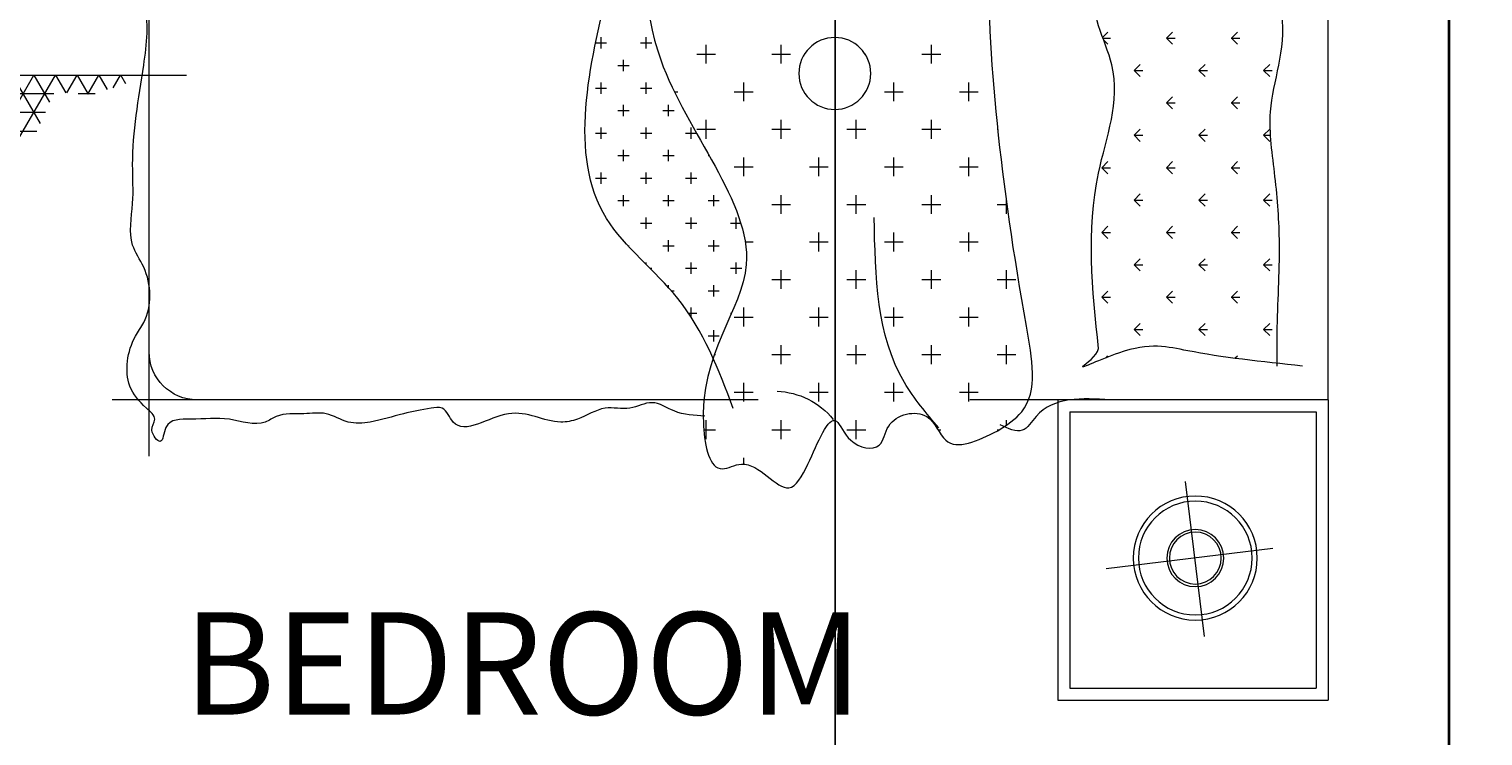
# Model space of a CAD drawing. Units: inches. Extents: x 3731 to 4318, y 1310 to 2388.
# Tile 17 of 57: x 4137 to 4237, y 1397 to 1445. Entities that reach past the tile are written whole.
import ezdxf

# ---------------------------------------------------------------- set-up
doc = ezdxf.new("R2010")
doc.units = ezdxf.units.IN
for name, color, linetype, lineweight in [('A-ANNO-DIMS', 2, 'Continuous', 18), ('A-AREA-IDEN', 7, 'Continuous', 18), ('A-FURN', 8, 'Continuous', 13), ('A-WALL', 7, 'Continuous', 35)]:
    doc.layers.add(name, color=color, linetype=linetype, lineweight=lineweight)
doc.styles.get("Standard").update_dxf_attribs({"font": 'arial.ttf'})
doc.dimstyles.get("Standard").update_dxf_attribs({"dimtxt": 0.18, "dimasz": 0.18, "dimexe": 0.18, "dimexo": 0.0625, "dimgap": 0.09, "dimtad": 0, "dimtih": 1, "dimtoh": 1, "dimdec": 4, "dimzin": 0, "dimdsep": 46, "dimtxsty": 'Standard', "dimcen": 0.09, "dimadec": 0, "dimazin": 0, "dimtfac": 1, "dimtdec": 4, "dimtofl": 0, "dimtmove": 0, "dimatfit": 3, "dimfxl": 1, "dimtolj": 1, "dimtzin": 0, "dimarcsym": 0})

# ---------------------------------------------------------------- blocks, each defined once
blk = doc.blocks.new('A$C200C7901')
for p, q in [((0, 1.8834), (0, 2.3334)), ((0.5, 2.3334), (0, 2.3334)), ((0.5, 2.3334), (0.5, 1.7369)), ((0.5, 2.3334), (0.5, 1.7369)), ((0.5, 2.3334), (2, 2.3334)), ((0.9943, 2.1721), (0.9842, 2.1822)), ((0.9943, 2.1721), (0.9842, 2.1822)), ((0.9943, 2.0643), (0.9842, 2.0744)), ((0.9943, 2.0643), (0.9842, 2.0744)), ((0.5701, 1.9635), (0.5733, 1.9666)), ((0.5701, 1.9635), (0.5733, 1.9666)), ((0.5, 1.8834), (0, 1.8834)), ((0.458, 1.7977), (0.466, 1.7977)), ((0.458, 1.7977), (0.466, 1.7977)), ((0.4504, 1.782), (0.4504, 1.7863)), ((0.4504, 1.782), (0.4504, 1.7863)), ((0.4504, 1.6834), (0.4504, 1.6883)), ((0.4504, 1.6834), (0.4504, 1.6883)), ((0.4656, 1.6727), (0.466, 1.6727)), ((0.4656, 1.6727), (0.466, 1.6727)), ((0.5597, 1.6727), (0.591, 1.6727)), ((0.5597, 1.6727), (0.591, 1.6727)), ((1.0129, 1.5945), (1.0129, 1.6258)), ((1.0129, 1.5945), (1.0129, 1.6258)), ((0.4504, 1.532), (0.4504, 1.5633)), ((1.0754, 1.5625), (1.0754, 1.5633)), ((1.0754, 1.5625), (1.0754, 1.5633)), ((0.4347, 1.5477), (0.466, 1.5477)), ((0.6847, 1.5477), (0.716, 1.5477)), ((0.4347, 1.4227), (0.466, 1.4227)), ((0.5, 1.3845), (0.5, 0.3086)), ((0.3931, 1.3602), (0.4035, 1.3602)), ((0.3931, 1.3602), (0.4035, 1.3602)), ((0.4972, 1.3602), (0.5285, 1.3602)), ((0.4972, 1.3602), (0.5285, 1.3602)), ((0.4504, 1.2936), (0.4504, 1.3133)), ((0.4504, 1.2936), (0.4504, 1.3133)), ((0.4347, 1.2977), (0.466, 1.2977)), ((0.4347, 1.2977), (0.466, 1.2977)), ((1.0407, 0.0275), (1.0407, 0.4323)), ((0.4061, 0.3703), (2.0386, 0.3703))]:
    blk.add_line(p, q)
at = {"linetype": 'ByBlock'}
for p, q in [((0.02, 1.9034), (0.02, 2.3134)), ((0.48, 2.3134), (0.02, 2.3134)), ((0.48, 1.9034), (0.48, 2.3134)), ((0.2524, 2.2412), (0.2186, 1.9635)), ((0.6171, 2.2259), (0.607, 2.236)), ((0.6171, 2.2259), (0.607, 2.236)), ((0.6171, 2.2259), (0.6171, 2.2402)), ((0.6171, 2.2259), (0.6171, 2.2402)), ((0.6171, 2.2259), (0.6272, 2.236)), ((0.6171, 2.2259), (0.6272, 2.236)), ((0.7249, 2.2259), (0.7148, 2.236)), ((0.7249, 2.2259), (0.7148, 2.236)), ((0.7249, 2.2259), (0.7249, 2.2402)), ((0.7249, 2.2259), (0.7249, 2.2402)), ((0.7249, 2.2259), (0.735, 2.236)), ((0.7249, 2.2259), (0.735, 2.236)), ((0.8326, 2.2259), (0.8225, 2.236)), ((0.8326, 2.2259), (0.8225, 2.236)), ((0.8326, 2.2259), (0.8326, 2.2402)), ((0.8326, 2.2259), (0.8326, 2.2402)), ((0.8326, 2.2259), (0.8427, 2.236)), ((0.8326, 2.2259), (0.8427, 2.236)), ((0.9404, 2.2259), (0.9303, 2.236)), ((0.9404, 2.2259), (0.9303, 2.236)), ((0.9404, 2.2259), (0.9404, 2.2369)), ((0.9404, 2.2259), (0.9404, 2.2369)), ((0.9404, 2.2259), (0.9505, 2.236)), ((0.9404, 2.2259), (0.9505, 2.236)), ((1.0482, 2.2259), (1.0381, 2.236)), ((1.0482, 2.2259), (1.0381, 2.236)), ((1.0482, 2.2259), (1.0482, 2.2402)), ((1.0482, 2.2259), (1.0482, 2.2402)), ((1.0482, 2.2259), (1.0583, 2.236)), ((1.0482, 2.2259), (1.0583, 2.236)), ((0.5692, 2.178), (0.5733, 2.1822)), ((0.5692, 2.178), (0.5733, 2.1822)), ((0.671, 2.1721), (0.6609, 2.1822)), ((0.671, 2.1721), (0.6609, 2.1822)), ((0.671, 2.172), (0.671, 2.1863)), ((0.671, 2.172), (0.671, 2.1863)), ((0.671, 2.1721), (0.6811, 2.1822)), ((0.671, 2.1721), (0.6811, 2.1822)), ((0.7787, 2.1721), (0.7686, 2.1822)), ((0.7787, 2.1721), (0.7686, 2.1822)), ((0.7787, 2.172), (0.7787, 2.1863)), ((0.7787, 2.172), (0.7787, 2.1863)), ((0.7787, 2.1721), (0.7889, 2.1822)), ((0.7787, 2.1721), (0.7889, 2.1822)), ((0.8865, 2.1721), (0.8764, 2.1822)), ((0.8865, 2.1721), (0.8764, 2.1822)), ((0.8865, 2.172), (0.8865, 2.1863)), ((0.8865, 2.172), (0.8865, 2.1863)), ((0.8865, 2.1721), (0.8966, 2.1822)), ((0.8865, 2.1721), (0.8966, 2.1822)), ((0.9943, 2.172), (0.9943, 2.1863)), ((0.9943, 2.172), (0.9943, 2.1863)), ((0.9943, 2.1721), (1.0044, 2.1822)), ((0.9943, 2.1721), (1.0044, 2.1822)), ((1.102, 2.1721), (1.0919, 2.1822)), ((1.102, 2.1721), (1.0919, 2.1822)), ((1.102, 2.172), (1.102, 2.1863)), ((1.102, 2.172), (1.102, 2.1863)), ((1.102, 2.1721), (1.1121, 2.1822)), ((1.102, 2.1721), (1.1121, 2.1822)), ((0.6171, 2.1182), (0.6171, 2.1325)), ((0.6171, 2.1182), (0.6171, 2.1325)), ((0.7249, 2.1182), (0.7249, 2.1325)), ((0.7249, 2.1182), (0.7249, 2.1325)), ((0.8326, 2.1182), (0.8326, 2.1325)), ((0.8326, 2.1182), (0.8326, 2.1325)), ((0.9404, 2.1182), (0.9404, 2.1325)), ((0.9404, 2.1182), (0.9404, 2.1325)), ((1.0482, 2.1182), (1.0482, 2.1325)), ((1.0482, 2.1182), (1.0482, 2.1325)), ((0.3641, 2.0951), (0.1061, 2.1268)), ((0.6171, 2.1182), (0.607, 2.1283)), ((0.6171, 2.1182), (0.607, 2.1283)), ((0.6171, 2.1182), (0.6272, 2.1283)), ((0.6171, 2.1182), (0.6272, 2.1283)), ((0.7249, 2.1182), (0.7148, 2.1283)), ((0.7249, 2.1182), (0.7148, 2.1283)), ((0.7249, 2.1182), (0.735, 2.1283)), ((0.7249, 2.1182), (0.735, 2.1283)), ((0.8326, 2.1182), (0.8225, 2.1283)), ((0.8326, 2.1182), (0.8225, 2.1283)), ((0.8326, 2.1182), (0.8427, 2.1283)), ((0.8326, 2.1182), (0.8427, 2.1283)), ((0.9404, 2.1182), (0.9303, 2.1283)), ((0.9404, 2.1182), (0.9303, 2.1283)), ((0.9404, 2.1182), (0.9505, 2.1283)), ((0.9404, 2.1182), (0.9505, 2.1283)), ((1.0482, 2.1182), (1.0381, 2.1283)), ((1.0482, 2.1182), (1.0381, 2.1283)), ((1.0482, 2.1182), (1.0583, 2.1283)), ((1.0482, 2.1182), (1.0583, 2.1283)), ((0.671, 2.0643), (0.6609, 2.0744)), ((0.671, 2.0643), (0.6609, 2.0744)), ((0.671, 2.0643), (0.671, 2.0786)), ((0.671, 2.0643), (0.671, 2.0786)), ((0.671, 2.0643), (0.6811, 2.0744)), ((0.671, 2.0643), (0.6811, 2.0744)), ((0.7787, 2.0643), (0.7686, 2.0744)), ((0.7787, 2.0643), (0.7686, 2.0744)), ((0.7787, 2.0643), (0.7787, 2.0786)), ((0.7787, 2.0643), (0.7787, 2.0786)), ((0.7787, 2.0643), (0.7889, 2.0744)), ((0.7787, 2.0643), (0.7889, 2.0744)), ((0.8865, 2.0643), (0.8764, 2.0744)), ((0.8865, 2.0643), (0.8764, 2.0744)), ((0.8865, 2.0643), (0.8865, 2.0786)), ((0.8865, 2.0643), (0.8865, 2.0786)), ((0.8865, 2.0643), (0.8966, 2.0744)), ((0.8865, 2.0643), (0.8966, 2.0744)), ((0.9943, 2.0643), (0.9943, 2.0786)), ((0.9943, 2.0643), (0.9943, 2.0786)), ((0.9943, 2.0643), (1.0044, 2.0744)), ((0.9943, 2.0643), (1.0044, 2.0744)), ((1.102, 2.0643), (1.0919, 2.0744)), ((1.102, 2.0643), (1.0919, 2.0744)), ((1.102, 2.0643), (1.102, 2.0786)), ((1.102, 2.0643), (1.102, 2.0786)), ((1.102, 2.0643), (1.1121, 2.0744)), ((1.102, 2.0643), (1.1121, 2.0744)), ((0.6171, 2.0104), (0.607, 2.0205)), ((0.6171, 2.0104), (0.607, 2.0205)), ((0.6171, 2.0104), (0.6171, 2.0247)), ((0.6171, 2.0104), (0.6171, 2.0247)), ((0.6171, 2.0104), (0.6272, 2.0205)), ((0.6171, 2.0104), (0.6272, 2.0205)), ((0.7249, 2.0104), (0.7148, 2.0205)), ((0.7249, 2.0104), (0.7148, 2.0205)), ((0.7249, 2.0104), (0.7249, 2.0247)), ((0.7249, 2.0104), (0.7249, 2.0247)), ((0.7249, 2.0104), (0.735, 2.0205)), ((0.7249, 2.0104), (0.735, 2.0205)), ((0.8326, 2.0104), (0.8225, 2.0205)), ((0.8326, 2.0104), (0.8225, 2.0205)), ((0.8326, 2.0104), (0.8326, 2.0247)), ((0.8326, 2.0104), (0.8326, 2.0247)), ((0.8326, 2.0104), (0.8427, 2.0205)), ((0.8326, 2.0104), (0.8427, 2.0205)), ((0.9404, 2.0104), (0.9303, 2.0205)), ((0.9404, 2.0104), (0.9303, 2.0205)), ((0.9404, 2.0104), (0.9404, 2.0247)), ((0.9404, 2.0104), (0.9404, 2.0247)), ((0.9404, 2.0104), (0.9505, 2.0205)), ((0.9404, 2.0104), (0.9505, 2.0205)), ((1.0482, 2.0104), (1.0381, 2.0205)), ((1.0482, 2.0104), (1.0381, 2.0205)), ((1.0482, 2.0104), (1.0482, 2.0247)), ((1.0482, 2.0104), (1.0482, 2.0247)), ((1.0482, 2.0104), (1.0583, 2.0205)), ((1.0482, 2.0104), (1.0583, 2.0205)), ((0.671, 1.9565), (0.6609, 1.9666)), ((0.671, 1.9565), (0.6609, 1.9666)), ((0.671, 1.9565), (0.671, 1.9708)), ((0.671, 1.9565), (0.671, 1.9708)), ((0.671, 1.9565), (0.6811, 1.9666)), ((0.671, 1.9565), (0.6811, 1.9666)), ((0.7787, 1.9565), (0.7686, 1.9666)), ((0.7787, 1.9565), (0.7686, 1.9666)), ((0.7787, 1.9565), (0.7787, 1.9708)), ((0.7787, 1.9565), (0.7787, 1.9708)), ((0.7787, 1.9565), (0.7889, 1.9666)), ((0.7787, 1.9565), (0.7889, 1.9666)), ((0.8865, 1.9565), (0.8764, 1.9666)), ((0.8865, 1.9565), (0.8764, 1.9666)), ((0.8865, 1.9565), (0.8865, 1.9708)), ((0.8865, 1.9565), (0.8865, 1.9708)), ((0.8865, 1.9565), (0.8966, 1.9666)), ((0.8865, 1.9565), (0.8966, 1.9666)), ((1.0993, 1.9593), (1.0919, 1.9666)), ((1.0993, 1.9593), (1.0919, 1.9666)), ((1.102, 1.9583), (1.102, 1.9708)), ((1.102, 1.9583), (1.102, 1.9708)), ((1.1033, 1.9578), (1.1121, 1.9666)), ((1.1033, 1.9578), (1.1121, 1.9666)), ((0.48, 1.9034), (0.02, 1.9034)), ((0.5597, 1.7977), (0.591, 1.7977)), ((0.5597, 1.7977), (0.591, 1.7977)), ((0.5754, 1.782), (0.5754, 1.8133)), ((0.5754, 1.782), (0.5754, 1.8133)), ((0.6847, 1.7977), (0.716, 1.7977)), ((0.6847, 1.7977), (0.716, 1.7977)), ((0.7004, 1.782), (0.7004, 1.8133)), ((0.7004, 1.782), (0.7004, 1.8133)), ((0.8097, 1.7977), (0.8331, 1.7977)), ((0.8097, 1.7977), (0.8331, 1.7977)), ((0.8254, 1.782), (0.8254, 1.7987)), ((0.8254, 1.782), (0.8254, 1.7987)), ((0.9504, 1.782), (0.9504, 1.7836)), ((0.9504, 1.782), (0.9504, 1.7836)), ((0.5129, 1.7195), (0.5129, 1.7508)), ((0.5129, 1.7195), (0.5129, 1.7508)), ((0.6379, 1.7195), (0.6379, 1.7508)), ((0.6379, 1.7195), (0.6379, 1.7508)), ((0.7629, 1.7195), (0.7629, 1.7508)), ((0.7629, 1.7195), (0.7629, 1.7508)), ((0.8879, 1.7195), (0.8879, 1.7508)), ((0.8879, 1.7195), (0.8879, 1.7508)), ((1.0129, 1.7195), (1.0129, 1.7508)), ((1.0129, 1.7195), (1.0129, 1.7508)), ((0.4972, 1.7352), (0.5285, 1.7352)), ((0.4972, 1.7352), (0.5285, 1.7352)), ((0.6222, 1.7352), (0.6535, 1.7352)), ((0.6222, 1.7352), (0.6535, 1.7352)), ((0.7472, 1.7352), (0.7785, 1.7352)), ((0.7472, 1.7352), (0.7785, 1.7352)), ((0.8722, 1.7352), (0.9035, 1.7352)), ((0.8722, 1.7352), (0.9035, 1.7352)), ((0.9972, 1.7352), (1.0285, 1.7352)), ((0.9972, 1.7352), (1.0285, 1.7352)), ((0.5754, 1.657), (0.5754, 1.6883)), ((0.5754, 1.657), (0.5754, 1.6883)), ((0.6847, 1.6727), (0.716, 1.6727)), ((0.6847, 1.6727), (0.716, 1.6727)), ((0.7004, 1.657), (0.7004, 1.6883)), ((0.7004, 1.657), (0.7004, 1.6883)), ((0.8097, 1.6727), (0.841, 1.6727)), ((0.8097, 1.6727), (0.841, 1.6727)), ((0.8254, 1.657), (0.8254, 1.6883)), ((0.8254, 1.657), (0.8254, 1.6883)), ((0.9347, 1.6727), (0.966, 1.6727)), ((0.9347, 1.6727), (0.966, 1.6727)), ((0.9504, 1.657), (0.9504, 1.6883)), ((0.9504, 1.657), (0.9504, 1.6883)), ((1.0597, 1.6727), (1.091, 1.6727)), ((1.0597, 1.6727), (1.091, 1.6727)), ((1.0754, 1.657), (1.0754, 1.6883)), ((1.0754, 1.657), (1.0754, 1.6883)), ((0.5129, 1.5945), (0.5129, 1.6258)), ((0.5129, 1.5945), (0.5129, 1.6258)), ((0.6379, 1.5945), (0.6379, 1.6258)), ((0.6379, 1.5945), (0.6379, 1.6258)), ((0.7629, 1.5945), (0.7629, 1.6258)), ((0.7629, 1.5945), (0.7629, 1.6258)), ((0.8879, 1.5945), (0.8879, 1.6258)), ((0.8879, 1.5945), (0.8879, 1.6258)), ((0.4972, 1.6102), (0.5285, 1.6102)), ((0.4972, 1.6102), (0.5285, 1.6102)), ((0.6222, 1.6102), (0.6535, 1.6102)), ((0.6222, 1.6102), (0.6535, 1.6102)), ((0.7472, 1.6102), (0.7785, 1.6102)), ((0.7472, 1.6102), (0.7785, 1.6102)), ((0.8722, 1.6102), (0.9035, 1.6102)), ((0.8722, 1.6102), (0.9035, 1.6102)), ((0.9972, 1.6102), (1.0285, 1.6102)), ((0.9972, 1.6102), (1.0285, 1.6102)), ((0.4504, 1.532), (0.4504, 1.5633)), ((0.5754, 1.532), (0.5754, 1.5633)), ((0.5754, 1.532), (0.5754, 1.5633)), ((0.7004, 1.532), (0.7004, 1.5633)), ((0.7004, 1.532), (0.7004, 1.5633)), ((0.8254, 1.532), (0.8254, 1.5633)), ((0.8254, 1.532), (0.8254, 1.5633)), ((0.9504, 1.532), (0.9504, 1.5633)), ((0.9504, 1.532), (0.9504, 1.5633)), ((0.4347, 1.5477), (0.466, 1.5477)), ((0.5597, 1.5477), (0.591, 1.5477)), ((0.5597, 1.5477), (0.591, 1.5477)), ((0.6847, 1.5477), (0.716, 1.5477)), ((0.8097, 1.5477), (0.841, 1.5477)), ((0.8097, 1.5477), (0.841, 1.5477)), ((0.9347, 1.5477), (0.966, 1.5477)), ((0.9347, 1.5477), (0.966, 1.5477)), ((0.5129, 1.4695), (0.5129, 1.5008)), ((0.5129, 1.4695), (0.5129, 1.5008)), ((0.6379, 1.4695), (0.6379, 1.5008)), ((0.6379, 1.4695), (0.6379, 1.5008)), ((0.7629, 1.4695), (0.7629, 1.5008)), ((0.7629, 1.4695), (0.7629, 1.5008)), ((0.8879, 1.4695), (0.8879, 1.5008)), ((0.8879, 1.4695), (0.8879, 1.5008)), ((0.4972, 1.4852), (0.5285, 1.4852)), ((0.4972, 1.4852), (0.5285, 1.4852)), ((0.6222, 1.4852), (0.6535, 1.4852)), ((0.6222, 1.4852), (0.6535, 1.4852)), ((0.7472, 1.4852), (0.7785, 1.4852)), ((0.7472, 1.4852), (0.7785, 1.4852)), ((0.8722, 1.4852), (0.9035, 1.4852)), ((0.8722, 1.4852), (0.9035, 1.4852)), ((0.4504, 1.407), (0.4504, 1.4383)), ((0.4504, 1.407), (0.4504, 1.4383)), ((0.5754, 1.407), (0.5754, 1.4383)), ((0.5754, 1.407), (0.5754, 1.4383)), ((0.7004, 1.407), (0.7004, 1.4383)), ((0.7004, 1.407), (0.7004, 1.4383)), ((0.8254, 1.407), (0.8254, 1.4383)), ((0.8254, 1.407), (0.8254, 1.4383)), ((0.9504, 1.407), (0.9504, 1.4383)), ((0.9504, 1.407), (0.9504, 1.4383)), ((1.0754, 1.407), (1.0754, 1.4383)), ((1.0754, 1.407), (1.0754, 1.4383)), ((0.4347, 1.4227), (0.466, 1.4227)), ((0.5597, 1.4227), (0.591, 1.4227)), ((0.5597, 1.4227), (0.591, 1.4227)), ((0.6847, 1.4227), (0.716, 1.4227)), ((0.6847, 1.4227), (0.716, 1.4227)), ((0.8097, 1.4227), (0.841, 1.4227)), ((0.8097, 1.4227), (0.841, 1.4227)), ((0.9347, 1.4227), (0.966, 1.4227)), ((0.9347, 1.4227), (0.966, 1.4227)), ((1.0597, 1.4227), (1.091, 1.4227)), ((1.0597, 1.4227), (1.091, 1.4227)), ((0.5129, 1.3445), (0.5129, 1.3758)), ((0.5129, 1.3445), (0.5129, 1.3758)), ((0.6222, 1.3602), (0.6535, 1.3602)), ((0.6222, 1.3602), (0.6535, 1.3602)), ((0.6379, 1.3445), (0.6379, 1.3758)), ((0.6379, 1.3445), (0.6379, 1.3758)), ((0.7191, 1.3383), (0.7191, 1.357)), ((0.7191, 1.3383), (0.7191, 1.357)), ((0.7629, 1.3627), (0.7629, 1.3758)), ((0.7629, 1.3627), (0.7629, 1.3758)), ((0.7762, 1.3602), (0.7785, 1.3602)), ((0.7762, 1.3602), (0.7785, 1.3602)), ((0.8722, 1.3602), (0.9035, 1.3602)), ((0.8722, 1.3602), (0.9035, 1.3602)), ((0.8879, 1.3445), (0.8879, 1.3758)), ((0.8879, 1.3445), (0.8879, 1.3758)), ((0.9972, 1.3602), (1.0285, 1.3602)), ((0.9972, 1.3602), (1.0285, 1.3602)), ((1.0129, 1.3445), (1.0129, 1.3758)), ((1.0129, 1.3445), (1.0129, 1.3758)), ((0.6441, 1.3383), (0.6441, 1.3399)), ((0.6441, 1.3383), (0.6441, 1.3399)), ((0.7097, 1.3477), (0.7285, 1.3477)), ((0.7097, 1.3477), (0.7285, 1.3477)), ((0.7847, 1.3477), (0.8035, 1.3477)), ((0.7847, 1.3477), (0.8035, 1.3477)), ((0.7941, 1.3383), (0.7941, 1.3554)), ((0.7941, 1.3383), (0.7941, 1.3554)), ((0.5754, 1.3115), (0.5754, 1.3133)), ((0.5754, 1.3115), (0.5754, 1.3133)), ((0.5972, 1.3102), (0.616, 1.3102)), ((0.5972, 1.3102), (0.616, 1.3102)), ((0.6066, 1.3008), (0.6066, 1.3195)), ((0.6066, 1.3008), (0.6066, 1.3195)), ((0.6722, 1.3102), (0.691, 1.3102)), ((0.6722, 1.3102), (0.691, 1.3102)), ((0.6816, 1.3008), (0.6816, 1.3195)), ((0.6816, 1.3008), (0.6816, 1.3195)), ((0.7472, 1.3102), (0.766, 1.3102)), ((0.7472, 1.3102), (0.766, 1.3102)), ((0.7566, 1.3008), (0.7566, 1.3195)), ((0.7566, 1.3008), (0.7566, 1.3195)), ((0.8222, 1.3102), (0.841, 1.3102)), ((0.8222, 1.3102), (0.841, 1.3102)), ((0.8316, 1.3008), (0.8316, 1.3195)), ((0.8316, 1.3008), (0.8316, 1.3195)), ((0.9504, 1.282), (0.9504, 1.3133)), ((0.9504, 1.282), (0.9504, 1.3133)), ((1.0754, 1.282), (1.0754, 1.3133)), ((1.0754, 1.282), (1.0754, 1.3133)), ((0.9066, 1.3008), (0.9066, 1.3028)), ((0.9066, 1.3008), (0.9066, 1.3028)), ((0.9347, 1.2977), (0.966, 1.2977)), ((0.9347, 1.2977), (0.966, 1.2977)), ((1.0597, 1.2977), (1.091, 1.2977)), ((1.0597, 1.2977), (1.091, 1.2977)), ((0.6379, 1.2727), (0.6535, 1.2727)), ((0.6379, 1.2727), (0.6535, 1.2727)), ((0.6441, 1.2686), (0.6441, 1.282)), ((0.6441, 1.2686), (0.6441, 1.282)), ((0.7097, 1.2727), (0.7285, 1.2727)), ((0.7097, 1.2727), (0.7285, 1.2727)), ((0.7191, 1.2633), (0.7191, 1.282)), ((0.7191, 1.2633), (0.7191, 1.282)), ((0.7847, 1.2727), (0.8035, 1.2727)), ((0.7847, 1.2727), (0.8035, 1.2727)), ((0.7941, 1.2633), (0.7941, 1.282)), ((0.7941, 1.2633), (0.7941, 1.282)), ((0.8597, 1.2727), (0.8785, 1.2727)), ((0.8597, 1.2727), (0.8785, 1.2727)), ((0.8691, 1.2633), (0.8691, 1.282)), ((0.8691, 1.2633), (0.8691, 1.282)), ((0.9347, 1.2727), (0.9535, 1.2727)), ((0.9347, 1.2727), (0.9535, 1.2727)), ((0.9441, 1.2633), (0.9441, 1.2816)), ((0.9441, 1.2633), (0.9441, 1.2816)), ((0.6816, 1.2398), (0.6816, 1.2445)), ((0.6816, 1.2398), (0.6816, 1.2445)), ((0.6868, 1.2352), (0.691, 1.2352)), ((0.6868, 1.2352), (0.691, 1.2352)), ((0.7472, 1.2352), (0.766, 1.2352)), ((0.7472, 1.2352), (0.766, 1.2352)), ((0.7566, 1.2258), (0.7566, 1.2445)), ((0.7566, 1.2258), (0.7566, 1.2445)), ((0.8222, 1.2352), (0.841, 1.2352)), ((0.8222, 1.2352), (0.841, 1.2352)), ((0.8316, 1.2258), (0.8316, 1.2445)), ((0.8316, 1.2258), (0.8316, 1.2445)), ((0.8972, 1.2352), (0.916, 1.2352)), ((0.8972, 1.2352), (0.916, 1.2352)), ((0.9066, 1.2258), (0.9066, 1.2445)), ((0.9066, 1.2258), (0.9066, 1.2445)), ((0.9722, 1.2352), (0.991, 1.2352)), ((0.9722, 1.2352), (0.991, 1.2352)), ((0.9816, 1.2258), (0.9816, 1.2445)), ((0.9816, 1.2258), (0.9816, 1.2445)), ((1.0129, 1.2448), (1.0129, 1.2508)), ((1.0129, 1.2448), (1.0129, 1.2508)), ((0.7191, 1.2041), (0.7191, 1.207)), ((0.7191, 1.2041), (0.7191, 1.207)), ((0.7255, 1.1977), (0.7285, 1.1977)), ((0.7255, 1.1977), (0.7285, 1.1977)), ((0.7847, 1.1977), (0.8035, 1.1977)), ((0.7847, 1.1977), (0.8035, 1.1977)), ((0.7941, 1.1883), (0.7941, 1.207)), ((0.7941, 1.1883), (0.7941, 1.207)), ((0.8597, 1.1977), (0.8785, 1.1977)), ((0.8597, 1.1977), (0.8785, 1.1977)), ((0.8691, 1.1883), (0.8691, 1.207)), ((0.8691, 1.1883), (0.8691, 1.207)), ((0.9347, 1.1977), (0.9535, 1.1977)), ((0.9347, 1.1977), (0.9535, 1.1977)), ((0.9441, 1.1883), (0.9441, 1.207)), ((0.9441, 1.1883), (0.9441, 1.207)), ((1.0097, 1.1977), (1.0285, 1.1977)), ((1.0097, 1.1977), (1.0285, 1.1977)), ((1.0191, 1.1883), (1.0191, 1.207)), ((1.0191, 1.1883), (1.0191, 1.207)), ((1.0847, 1.1977), (1.1035, 1.1977)), ((1.0847, 1.1977), (1.1035, 1.1977)), ((1.0941, 1.1883), (1.0941, 1.207)), ((1.0941, 1.1883), (1.0941, 1.207)), ((0.7566, 1.1674), (0.7566, 1.1695)), ((0.7566, 1.1674), (0.7566, 1.1695)), ((0.8316, 1.1508), (0.8316, 1.1695)), ((0.8316, 1.1508), (0.8316, 1.1695)), ((0.9066, 1.1508), (0.9066, 1.1695)), ((0.9066, 1.1508), (0.9066, 1.1695)), ((0.9816, 1.1508), (0.9816, 1.1695)), ((0.9816, 1.1508), (0.9816, 1.1695)), ((1.0566, 1.1508), (1.0566, 1.1695)), ((1.0566, 1.1508), (1.0566, 1.1695)), ((0.7646, 1.1602), (0.766, 1.1602)), ((0.7646, 1.1602), (0.766, 1.1602)), ((0.8222, 1.1602), (0.841, 1.1602)), ((0.8222, 1.1602), (0.841, 1.1602)), ((0.8972, 1.1602), (0.916, 1.1602)), ((0.8972, 1.1602), (0.916, 1.1602)), ((0.9722, 1.1602), (0.991, 1.1602)), ((0.9722, 1.1602), (0.991, 1.1602)), ((1.0472, 1.1602), (1.066, 1.1602)), ((1.0472, 1.1602), (1.066, 1.1602)), ((0.8597, 1.1227), (0.8785, 1.1227)), ((0.8597, 1.1227), (0.8785, 1.1227)), ((0.8691, 1.1133), (0.8691, 1.132)), ((0.8691, 1.1133), (0.8691, 1.132)), ((0.9347, 1.1227), (0.9535, 1.1227)), ((0.9347, 1.1227), (0.9535, 1.1227)), ((0.9441, 1.1133), (0.9441, 1.132)), ((0.9441, 1.1133), (0.9441, 1.132)), ((1.0097, 1.1227), (1.0285, 1.1227)), ((1.0097, 1.1227), (1.0285, 1.1227)), ((1.0191, 1.1133), (1.0191, 1.132)), ((1.0191, 1.1133), (1.0191, 1.132)), ((1.0847, 1.1227), (1.1035, 1.1227)), ((1.0847, 1.1227), (1.1035, 1.1227)), ((1.0941, 1.1136), (1.0941, 1.132)), ((1.0941, 1.1136), (1.0941, 1.132)), ((1.0194, 0.3103), (1.0407, 0.3227)), ((1.0194, 0.3103), (1.0407, 0.3227)), ((1.0261, 0.3316), (1.0407, 0.3232)), ((1.0261, 0.3316), (1.0407, 0.3232)), ((1.0164, 0.3011), (1.0407, 0.2871)), ((1.0164, 0.3011), (1.0407, 0.2871)), ((1.0088, 0.2694), (1.0407, 0.251)), ((1.0088, 0.2694), (1.0407, 0.251)), ((1.0089, 0.2682), (1.0407, 0.2866)), ((1.0089, 0.2682), (1.0407, 0.2866)), ((1.0099, 0.2521), (1.0099, 0.2804)), ((1.0099, 0.2521), (1.0099, 0.2804)), ((1.0111, 0.2334), (1.0407, 0.2505)), ((1.0111, 0.2334), (1.0407, 0.2505)), ((1.0112, 0.232), (1.0407, 0.215)), ((1.0112, 0.232), (1.0407, 0.215)), ((0.9344, 0.153), (1.0407, 0.2144)), ((0.9344, 0.153), (1.0407, 0.2144)), ((0.9787, 0.0381), (0.9787, 0.1976)), ((0.9787, 0.0381), (0.9787, 0.1976)), ((0.9953, 0.2051), (1.0407, 0.1789)), ((0.9953, 0.2051), (1.0407, 0.1789)), ((1.0099, 0.0251), (1.0099, 0.2117)), ((1.0099, 0.0251), (1.0099, 0.2117)), ((0.9355, 0.1176), (1.0407, 0.1783)), ((0.9355, 0.1176), (1.0407, 0.1783)), ((0.9474, 0.0512), (0.9474, 0.1835)), ((0.9474, 0.0512), (0.9474, 0.1835)), ((0.9602, 0.1893), (1.0407, 0.1428)), ((0.9602, 0.1893), (1.0407, 0.1428))]:
    blk.add_line(p, q, dxfattribs=at)
for radius in [0.1032, 0.0947, 0.0475, 0.0432]:
    blk.add_circle((0.2367, 2.1121), radius, dxfattribs=at)
blk.add_circle((1.0433, 1.5119), 0.0599)
blk.add_arc((0.3888, 1.4113), 0.1256, 1.9962, 51.1646, dxfattribs=at)
for centre, radius, start, end in [((0.3888, 1.4113), 0.1256, 1.9962, 51.1646), ((0.58, 0.4503), 0.08, 180, 270)]:
    blk.add_arc(centre, radius, start, end)
for points, knots in [([(0.5562, 2.2908), (0.5634, 2.223), (0.5751, 2.1147), (0.6005, 2.0213), (0.5392, 1.8966), (0.5726, 1.9486), (0.5854, 1.951)], [0, 0, 0, 0, 193.119101, 308.278592, 371.468985, 410.593498, 410.593498, 410.593498, 410.593498]), ([(0.5854, 1.951), (0.6835, 1.9407), (0.8425, 1.9242), (1.0374, 2.0054), (1.1564, 1.9255), (1.2274, 1.9841), (1.2052, 2.0751), (1.1815, 2.152), (1.2176, 2.2368), (1.0992, 2.2731), (1.0008, 2.2255), (0.8698, 2.246), (0.7481, 2.2548), (0.6426, 2.2473), (0.5746, 2.2478), (0.5562, 2.2479)], [0, 0, 0, 0, 292.165466, 473.33038, 601.631673, 630.723769, 727.138505, 836.819956, 887.958136, 954.42438, 1118.989809, 1227.016542, 1338.750986, 1487.447361, 1542.751028, 1542.751028, 1542.751028, 1542.751028]), ([(0.4485, 1.7835), (0.4321, 1.7496), (0.4062, 1.6964), (0.49, 1.6713), (0.4719, 1.5969), (0.4123, 1.592), (0.4233, 1.5337), (0.4954, 1.5086), (0.4012, 1.4738), (0.3253, 1.4306), (0.4113, 1.3764), (0.3688, 1.3065), (0.5579, 1.2663), (0.741, 1.4533), (1.1127, 1.1109), (1.4811, 1.2478), (1.7885, 1.3492), (2.0357, 1.1637), (2.0748, 1.2974), (2.0876, 1.349), (2.0192, 1.3805), (2.0564, 1.4298), (2.0588, 1.4846), (1.9759, 1.5349), (2.1004, 1.5845), (2.0397, 1.6519), (1.971, 1.7053), (2.1104, 1.8981), (1.5946, 1.7967), (1.2448, 1.7472), (0.8129, 1.7935), (0.4953, 1.8548), (0.4582, 1.7983), (0.4485, 1.7835)], [0, 0, 0, 0, 88.420092, 139.08588, 204.302936, 239.695496, 287.801042, 327.365471, 412.960499, 463.626286, 552.059846, 584.668336, 662.614915, 940.993281, 1309.926334, 1844.022653, 1996.276242, 2316.43048, 2341.441004, 2404.707416, 2449.463774, 2514.680778, 2538.40571, 2613.031547, 2697.13096, 2760.903931, 2822.692699, 2945.47, 3215.060018, 3725.584917, 4361.974444, 4504.671998, 4555.32777, 4555.32777, 4555.32777, 4555.32777]), ([(0.4856, 1.3429), (0.5504, 1.3182), (0.6715, 1.2721), (0.8374, 1.0498), (1.1164, 1.1183), (1.3878, 1.1816), (1.5888, 1.1102), (1.8403, 1.1127), (1.9415, 1.2178), (2.0032, 1.2819)], [0, 0, 0, 0, 205.411753, 383.654933, 772.067458, 921.644661, 1226.793228, 1388.983508, 1642.292305, 1642.292305, 1642.292305, 1642.292305])]:
    blk.add_open_spline(points, degree=3, knots=knots)
for points, knots in [([(0.5, 1.9703), (0.5029, 1.9235), (0.5066, 1.8648), (0.4398, 1.8252), (0.452, 1.8005), (0.4585, 1.7872)], [0, 0, 0, 0, 126.315232, 158.854004, 196.789047, 196.789047, 196.789047, 196.789047]), ([(0.5, 1.9703), (0.5029, 1.9235), (0.5066, 1.8648), (0.4398, 1.8252), (0.452, 1.8005), (0.4585, 1.7872)], [0, 0, 0, 0, 126.315232, 158.854004, 196.789047, 196.789047, 196.789047, 196.789047]), ([(0.4532, 1.6853), (0.4776, 1.6644), (0.574, 1.582), (0.7055, 1.5794), (0.8037, 1.5774)], [0, 0, 0, 0, 94.920667, 374.457292, 374.457292, 374.457292, 374.457292]), ([(0.4532, 1.6853), (0.4776, 1.6644), (0.574, 1.582), (0.7055, 1.5794), (0.8037, 1.5774)], [0, 0, 0, 0, 94.920667, 374.457292, 374.457292, 374.457292, 374.457292]), ([(0.473, 1.2954), (0.4739, 1.2781), (0.4755, 1.2477), (0.5032, 1.2084), (0.4801, 1.1701), (0.4928, 1.1255), (0.4674, 1.0912), (0.4579, 1.0351), (0.501, 0.9724), (0.4311, 0.8832), (0.4902, 0.8637), (0.4843, 0.8288), (0.4774, 0.7906), (0.4625, 0.7457), (0.459, 0.6999), (0.4816, 0.6664), (0.4748, 0.625), (0.4791, 0.5889), (0.4533, 0.5528), (0.4738, 0.5004), (0.4658, 0.4502), (0.4696, 0.3946), (0.4189, 0.3935), (0.4493, 0.3684), (0.4694, 0.3857), (0.4922, 0.3576), (0.5297, 0.3262), (0.5917, 0.3353), (0.6454, 0.3754), (0.7083, 0.3741), (0.7643, 0.3328), (0.826, 0.346), (0.925, 0.3388), (1.0353, 0.3593), (1.1561, 0.3744), (1.2477, 0.3154), (1.3302, 0.3474), (1.4086, 0.3512), (1.5217, 0.3878), (1.6362, 0.3176), (1.7682, 0.3285), (1.8402, 0.3019), (1.9071, 0.3529), (1.9647, 0.3412), (2.0795, 0.2948), (2.0472, 0.3498), (2.0343, 0.3772), (2.0435, 0.43), (2.0109, 0.5782), (2.0746, 0.4643), (2.0805, 0.584), (2.0084, 0.5979), (2.0343, 0.6846), (2.0344, 0.746), (2.0293, 0.8096), (2.0489, 0.8545), (2.0652, 0.9218), (1.9842, 0.9297), (2.0007, 1.0162), (2.0367, 1.0585), (2.0367, 1.1102), (2.0457, 1.1647), (2.0226, 1.2084), (2.0234, 1.2306), (2.0236, 1.2352)], [0, 0, 0, 0, 51.660678, 90.967412, 128.902454, 170.303599, 219.852997, 247.834962, 336.321557, 429.35469, 458.821847, 477.222321, 524.135809, 581.038434, 617.839381, 657.146115, 693.947125, 740.178081, 760.753248, 820.731705, 885.133458, 928.777044, 953.563729, 976.574207, 995.553042, 1018.563482, 1064.584401, 1147.951297, 1174.787598, 1266.851571, 1308.018447, 1377.066427, 1441.511314, 1608.245014, 1714.11869, 1792.771707, 1913.247991, 1954.931389, 2029.864445, 2259.189419, 2305.221512, 2429.507982, 2456.344283, 2543.92595, 2627.925037, 2662.96218, 2687.736879, 2719.937755, 2839.540991, 2875.47895, 2953.681041, 2993.270313, 3066.872333, 3154.395764, 3200.397042, 3248.426375, 3312.828127, 3347.881398, 3444.484026, 3481.577522, 3518.665244, 3592.267265, 3644.719162, 3658.519501, 3658.519501, 3658.519501, 3658.519501])]:
    blk.add_open_spline(points, degree=3, knots=knots, dxfattribs=at)
blk = doc.blocks.new('*D32')
at = {"layer": 'A-ANNO-DIMS', "color": 0, "lineweight": -2, "transparency": 16777216}
for p, q in [((4269.211, 1592.319), (4269.211, 1310.251)), ((3835.209, 1359.319), (3835.209, 1310.251)), ((3835.389, 1310.431), (4051.918, 1310.431)), ((4269.031, 1310.431), (4052.502, 1310.431))]:
    blk.add_line(p, q, dxfattribs=at)
at = {"layer": 'A-ANNO-DIMS', "color": 0, "transparency": 16777216}
for points in [[(3835.389, 1310.461), (3835.389, 1310.401), (3835.209, 1310.431)], [(4269.031, 1310.461), (4269.031, 1310.401), (4269.211, 1310.431)]]:
    blk.add_solid(points, dxfattribs=at)
at = {"layer": 'Defpoints', "color": 0, "transparency": 16777216}
for p in [(4269.211, 1592.382), (3835.209, 1359.382), (4269.211, 1310.431)]:
    blk.add_point(p, dxfattribs=at)
at = {"layer": 'A-ANNO-DIMS', "color": 0, "transparency": 16777216, "insert": (4052.21, 1310.431), "char_height": 0.18, "attachment_point": 5}
blk.add_mtext('\\A1;434', dxfattribs=at)
blk = doc.blocks.new('*D46')
at = {"layer": 'A-ANNO-DIMS', "color": 0, "lineweight": -2, "transparency": 16777216}
for p, q in [((4112.209, 1854.319), (4112.209, 1310.251)), ((4192.209, 1854.319), (4192.209, 1310.251)), ((4112.389, 1310.431), (4151.99, 1310.431)), ((4192.029, 1310.431), (4152.428, 1310.431))]:
    blk.add_line(p, q, dxfattribs=at)
at = {"layer": 'A-ANNO-DIMS', "color": 0, "transparency": 16777216}
for points in [[(4112.389, 1310.461), (4112.389, 1310.401), (4112.209, 1310.431)], [(4192.029, 1310.461), (4192.029, 1310.401), (4192.209, 1310.431)]]:
    blk.add_solid(points, dxfattribs=at)
at = {"layer": 'Defpoints', "color": 0, "transparency": 16777216}
for p in [(4112.209, 1854.382), (4192.209, 1854.382), (4192.209, 1310.431)]:
    blk.add_point(p, dxfattribs=at)
at = {"layer": 'A-ANNO-DIMS', "color": 0, "transparency": 16777216, "insert": (4152.209, 1310.431), "char_height": 0.18, "attachment_point": 5}
blk.add_mtext('\\A1;80', dxfattribs=at)
blk = doc.blocks.new('*D47')
at = {"layer": 'A-ANNO-DIMS', "color": 0, "lineweight": -2, "transparency": 16777216}
for p, q in [((4192.209, 1854.319), (4192.209, 1310.251)), ((4234.209, 1854.319), (4234.209, 1310.251)), ((4192.389, 1310.431), (4212.987, 1310.431)), ((4234.029, 1310.431), (4213.43, 1310.431))]:
    blk.add_line(p, q, dxfattribs=at)
at = {"layer": 'A-ANNO-DIMS', "color": 0, "transparency": 16777216}
for points in [[(4192.389, 1310.461), (4192.389, 1310.401), (4192.209, 1310.431)], [(4234.029, 1310.461), (4234.029, 1310.401), (4234.209, 1310.431)]]:
    blk.add_solid(points, dxfattribs=at)
at = {"layer": 'Defpoints', "color": 0, "transparency": 16777216}
for p in [(4192.209, 1854.382), (4234.209, 1854.382), (4234.209, 1310.431)]:
    blk.add_point(p, dxfattribs=at)
at = {"layer": 'A-ANNO-DIMS', "color": 0, "transparency": 16777216, "insert": (4213.209, 1310.431), "char_height": 0.18, "attachment_point": 5}
blk.add_mtext('\\A1;42', dxfattribs=at)

msp = doc.modelspace()

# ---------------------------------------------------------------- linework, layer by layer
at = {"layer": 'A-WALL'}
msp.add_line((4234.211, 1527.382), (4234.211, 1364.382), dxfattribs=at)

# ---------------------------------------------------------------- block references
at = {"layer": 'A-FURN', "xscale": -41.1071563136412, "yscale": 41.1071563136412, "zscale": 41.1071563136412, "rotation": 270}
msp.add_blockref('A$C200C7901', (4130.025, 1399.263), dxfattribs=at)

# ---------------------------------------------------------------- texts
at = {"layer": 'A-AREA-IDEN', "insert": (4147.599, 1405.281), "char_height": 7, "attachment_point": 1}
msp.add_mtext_dynamic_manual_height_columns('BEDROOM\\P10\'-0"X13\'-3"', width=47.04372, gutter_width=12.5, heights=[0], dxfattribs=at)

# ---------------------------------------------------------------- dimensions: what is measured, and where the dimension line sits
at = {"layer": 'A-ANNO-DIMS'}
for base, p1, p2, picture, middle in [((4192.209, 1310.431), (4112.209, 1854.382), (4192.209, 1854.382), '*D46', (4152.209, 1310.431)), ((4234.209, 1310.431), (4192.209, 1854.382), (4234.209, 1854.382), '*D47', (4213.209, 1310.431)), ((4269.211, 1310.431), (3835.209, 1359.382), (4269.211, 1592.382), '*D32', (4052.21, 1310.431))]:
    dim = msp.add_linear_dim(base=base, p1=p1, p2=p2, dimstyle='Standard', override={"dimdec": 0, "dimlfac": 1, "dimrnd": 0, "dimzin": 0, "dimdsep": 46, "dimlunit": 2}, dxfattribs=at)
    dim.commit()
    dim.dimension.update_dxf_attribs({"geometry": picture, "text_midpoint": middle})

doc.saveas('drawing.dxf')
